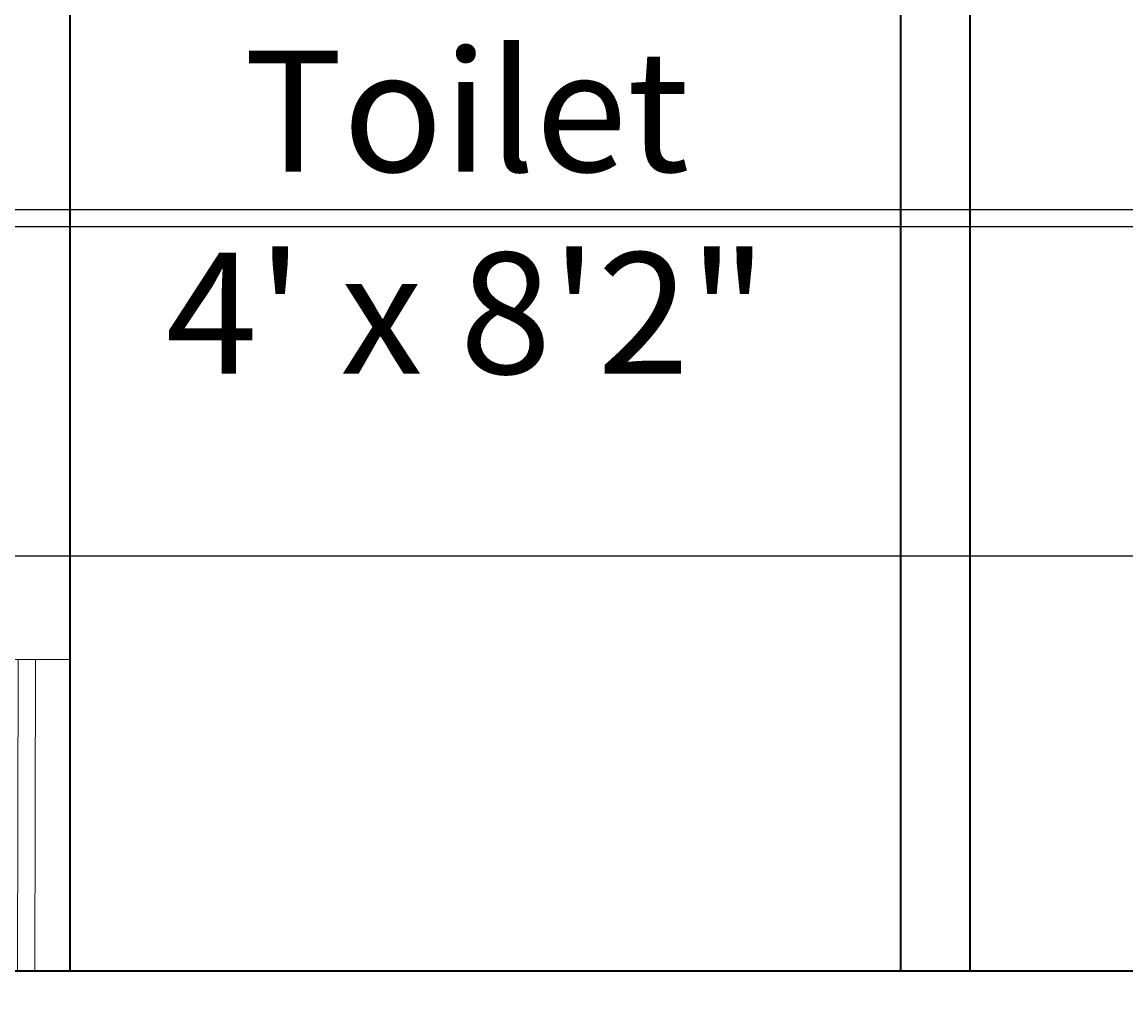
# Model space of a CAD drawing. Units: feet. Extents: x 105 to 1094, y -88 to 588.
# Tile 19 of 59: x 372 to 436, y 250 to 307. Entities that reach past the tile are written whole.
import ezdxf

# ---------------------------------------------------------------- set-up
doc = ezdxf.new("R2010")
doc.units = ezdxf.units.FT
doc.header["$MEASUREMENT"] = 0
for name, color, linetype, lineweight in [('A-ANNO-DIMS', 2, 'Continuous', 18), ('A-AREA-IDEN', 7, 'Continuous', 18), ('A-GLAZ', 4, 'Continuous', 18), ('A-WALL', 7, 'Continuous', 35)]:
    doc.layers.add(name, color=color, linetype=linetype, lineweight=lineweight)
doc.styles.get("Standard").update_dxf_attribs({"font": 'arial.ttf'})
doc.dimstyles.get("Standard").update_dxf_attribs({"dimtxt": 0.18, "dimasz": 0.18, "dimexe": 0.18, "dimexo": 0.0625, "dimgap": 0.09, "dimtad": 0, "dimtih": 1, "dimtoh": 1, "dimdec": 4, "dimzin": 0, "dimdsep": 46, "dimtxsty": 'Standard', "dimcen": 0.09, "dimadec": 0, "dimazin": 0, "dimtfac": 1, "dimtdec": 4, "dimtofl": 0, "dimtmove": 0, "dimatfit": 3, "dimfxl": 1, "dimtolj": 1, "dimtzin": 0, "dimarcsym": 0})

# ---------------------------------------------------------------- blocks, each defined once
blk = doc.blocks.new('VENT-LONGITUDINAL')
for p, q in [((0, 18), (4, 18)), ((2.039, 0), (2, 18)), ((3.039, 0.002), (3, 18.002))]:
    blk.add_line(p, q)
blk = doc.blocks.new('*D20')
at = {"layer": 'A-ANNO-DIMS', "color": 0, "lineweight": -2, "transparency": 16777216}
for p, q in [((150.688, 276.019), (150.688, -88.149)), ((1048.688, 276.019), (1048.688, -88.149)), ((150.868, -87.969), (599.399, -87.969)), ((1048.508, -87.969), (599.977, -87.969))]:
    blk.add_line(p, q, dxfattribs=at)
at = {"layer": 'A-ANNO-DIMS', "color": 0, "transparency": 16777216}
for points in [[(150.868, -87.939), (150.868, -87.999), (150.688, -87.969)], [(1048.508, -87.939), (1048.508, -87.999), (1048.688, -87.969)]]:
    blk.add_solid(points, dxfattribs=at)
at = {"layer": 'Defpoints', "color": 0, "transparency": 16777216}
for p in [(150.688, 276.081), (1048.688, 276.081), (1048.688, -87.969)]:
    blk.add_point(p, dxfattribs=at)
at = {"layer": 'A-ANNO-DIMS', "color": 0, "transparency": 16777216, "insert": (599.688, -87.969), "char_height": 0.18, "attachment_point": 5}
blk.add_mtext('\\A1;898', dxfattribs=at)
blk = doc.blocks.new('*D21')
at = {"layer": 'A-ANNO-DIMS', "color": 0, "lineweight": -2, "transparency": 16777216}
for p, q in [((849.626, 543.081), (105.458, 543.081)), ((105.638, 542.901), (105.638, 250.263)), ((105.638, -42.739), (105.638, 249.899)), ((849.626, -42.919), (105.458, -42.919))]:
    blk.add_line(p, q, dxfattribs=at)
at = {"layer": 'A-ANNO-DIMS', "color": 0, "transparency": 16777216}
for points in [[(105.608, 542.901), (105.668, 542.901), (105.638, 543.081)], [(105.608, -42.739), (105.668, -42.739), (105.638, -42.919)]]:
    blk.add_solid(points, dxfattribs=at)
at = {"layer": 'Defpoints', "color": 0, "transparency": 16777216}
for p in [(105.638, 543.081), (849.688, 543.081), (849.688, -42.919)]:
    blk.add_point(p, dxfattribs=at)
at = {"layer": 'A-ANNO-DIMS', "color": 0, "transparency": 16777216, "insert": (105.638, 250.081), "char_height": 0.18, "attachment_point": 5}
blk.add_mtext('\\A1;586', dxfattribs=at)
blk = doc.blocks.new('*D33')
at = {"layer": 'A-ANNO-DIMS', "color": 0, "lineweight": -2, "transparency": 16777216}
for p, q in [((646.626, 395.081), (105.458, 395.081)), ((105.638, 394.901), (105.638, 345.263)), ((105.638, 295.261), (105.638, 344.899)), ((646.626, 295.081), (105.458, 295.081))]:
    blk.add_line(p, q, dxfattribs=at)
at = {"layer": 'A-ANNO-DIMS', "color": 0, "transparency": 16777216}
for points in [[(105.608, 394.901), (105.668, 394.901), (105.638, 395.081)], [(105.608, 295.261), (105.668, 295.261), (105.638, 295.081)]]:
    blk.add_solid(points, dxfattribs=at)
at = {"layer": 'Defpoints', "color": 0, "transparency": 16777216}
for p in [(646.688, 395.081), (105.638, 295.081), (646.688, 295.081)]:
    blk.add_point(p, dxfattribs=at)
at = {"layer": 'A-ANNO-DIMS', "color": 0, "transparency": 16777216, "insert": (105.638, 345.081), "char_height": 0.18, "attachment_point": 5}
blk.add_mtext('\\A1;100', dxfattribs=at)
blk = doc.blocks.new('*D54')
at = {"layer": 'A-ANNO-DIMS', "color": 0, "lineweight": -2, "transparency": 16777216}
for p, q in [((294.751, 296.081), (1093.918, 296.081)), ((1093.738, 295.901), (1093.738, 286.263)), ((1093.738, 276.261), (1093.738, 285.899)), ((294.751, 276.081), (1093.918, 276.081))]:
    blk.add_line(p, q, dxfattribs=at)
at = {"layer": 'A-ANNO-DIMS', "color": 0, "transparency": 16777216}
for points in [[(1093.708, 295.901), (1093.768, 295.901), (1093.738, 296.081)], [(1093.708, 276.261), (1093.768, 276.261), (1093.738, 276.081)]]:
    blk.add_solid(points, dxfattribs=at)
at = {"layer": 'Defpoints', "color": 0, "transparency": 16777216}
for p in [(294.688, 296.081), (1093.738, 296.081), (294.688, 276.081)]:
    blk.add_point(p, dxfattribs=at)
at = {"layer": 'A-ANNO-DIMS', "color": 0, "transparency": 16777216, "insert": (1093.738, 286.081), "char_height": 0.18, "attachment_point": 5}
blk.add_mtext('\\A1;20', dxfattribs=at)
blk = doc.blocks.new('*D56')
at = {"layer": 'A-ANNO-DIMS', "color": 0, "lineweight": -2, "transparency": 16777216}
for p, q in [((374.688, 252.144), (374.688, 588.311)), ((374.868, 588.131), (398.466, 588.131)), ((422.508, 588.131), (398.911, 588.131)), ((422.688, 252.144), (422.688, 588.311))]:
    blk.add_line(p, q, dxfattribs=at)
at = {"layer": 'A-ANNO-DIMS', "color": 0, "transparency": 16777216}
for points in [[(374.868, 588.161), (374.868, 588.101), (374.688, 588.131)], [(422.508, 588.161), (422.508, 588.101), (422.688, 588.131)]]:
    blk.add_solid(points, dxfattribs=at)
at = {"layer": 'Defpoints', "color": 0, "transparency": 16777216}
for p in [(422.688, 588.131), (374.688, 252.081), (422.688, 252.081)]:
    blk.add_point(p, dxfattribs=at)
at = {"layer": 'A-ANNO-DIMS', "color": 0, "transparency": 16777216, "insert": (398.688, 588.131), "char_height": 0.18, "attachment_point": 5}
blk.add_mtext('\\A1;48', dxfattribs=at)

msp = doc.modelspace()

# ---------------------------------------------------------------- linework, layer by layer
at = {"layer": 'A-WALL'}
for p, q in [((374.6883, 252.0812), (374.6883, 354.0812)), ((426.6883, 252.0812), (426.6883, 354.0812)), ((422.6883, 252.0812), (422.6883, 350.0812)), ((422.6883, 252.0812), (370.6883, 252.0812)), ((552.6883, 252.0812), (370.6883, 252.0812)), ((552.6883, 252.0812), (426.6883, 252.0812))]:
    msp.add_line(p, q, dxfattribs=at)

# ---------------------------------------------------------------- block references
at = {"layer": 'A-GLAZ', "extrusion": (0, 0, -1), "zscale": -1}
msp.add_blockref('VENT-LONGITUDINAL', (-374.6886, 252.081), dxfattribs=at)

# ---------------------------------------------------------------- texts
at = {"layer": 'A-AREA-IDEN', "insert": (446.7646, 305.2595), "char_height": 7, "attachment_point": 3}
msp.add_mtext_dynamic_manual_height_columns('\\pxqc;Toilet \\P4\' x 8\'2"', width=98.34246, gutter_width=1, heights=[0], dxfattribs=at)

# ---------------------------------------------------------------- dimensions: what is measured, and where the dimension line sits
at = {"layer": 'A-ANNO-DIMS'}
for base, p1, p2, picture, middle in [((422.6883, 588.1312), (374.6883, 252.0812), (422.6883, 252.0812), '*D56', (398.6883, 588.1312)), ((1048.6883, -87.9688), (150.6883, 276.0812), (1048.6883, 276.0812), '*D20', (599.6883, -87.9688))]:
    dim = msp.add_linear_dim(base=base, p1=p1, p2=p2, dimstyle='Standard', override={"dimdec": 0, "dimlfac": 1, "dimrnd": 0, "dimzin": 0, "dimdsep": 46, "dimlunit": 2}, dxfattribs=at)
    dim.commit()
    dim.dimension.update_dxf_attribs({"geometry": picture, "text_midpoint": middle})
for base, p1, p2, picture, middle in [((105.6383, 543.0812), (849.6883, -42.9188), (849.6883, 543.0812), '*D21', (105.6383, 250.0812)), ((105.6383, 295.0812), (646.6883, 395.0812), (646.6883, 295.0812), '*D33', (105.6383, 345.0812)), ((1093.7383, 296.0812), (294.6883, 276.0812), (294.6883, 296.0812), '*D54', (1093.7383, 286.0812))]:
    dim = msp.add_linear_dim(base=base, p1=p1, p2=p2, angle=90, dimstyle='Standard', override={"dimdec": 0, "dimlfac": 1, "dimrnd": 0, "dimzin": 0, "dimdsep": 46, "dimlunit": 2}, dxfattribs=at)
    dim.commit()
    dim.dimension.update_dxf_attribs({"geometry": picture, "text_midpoint": middle})

doc.saveas('drawing.dxf')
